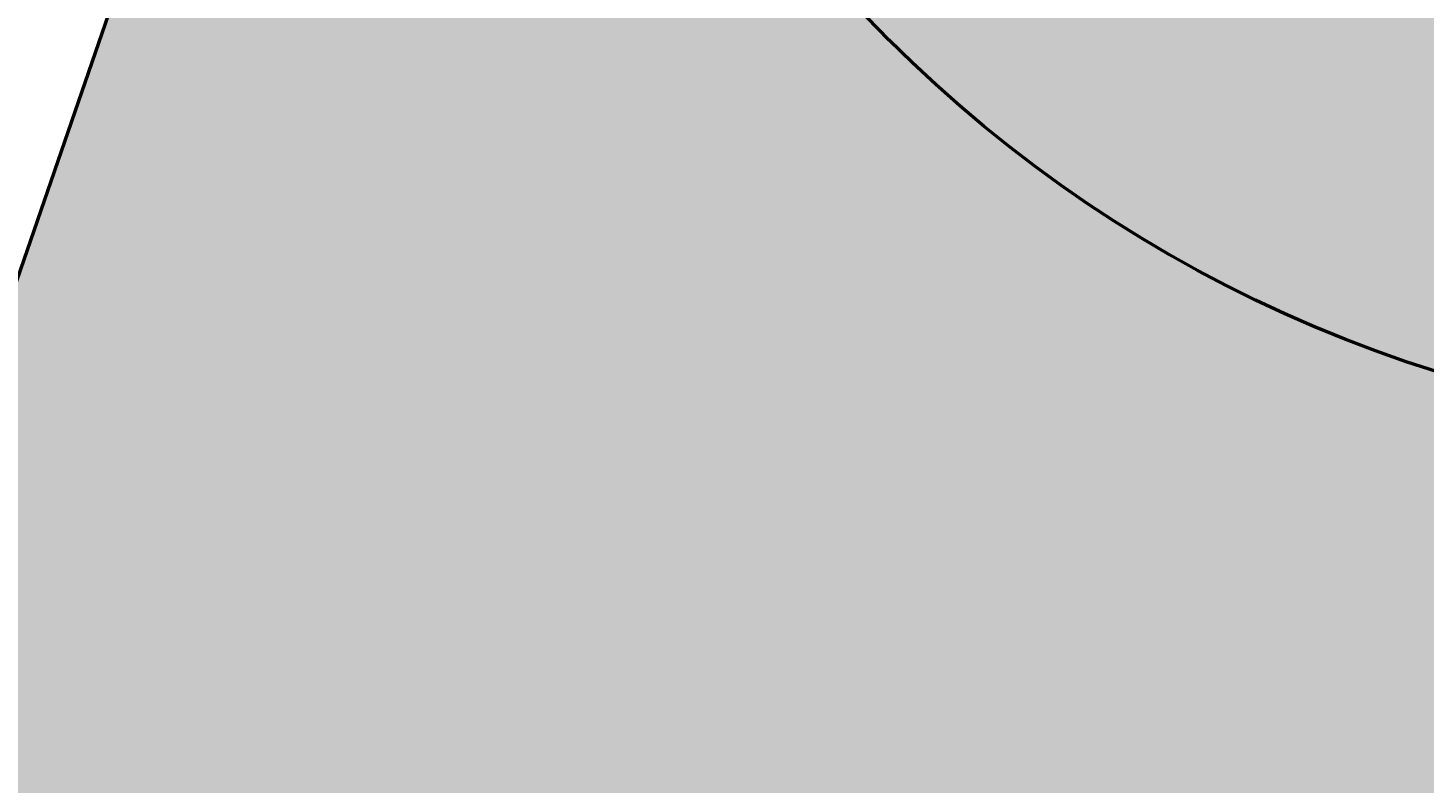
# Model space of a CAD drawing. Units: inches. Extents: x 114 to 236, y -51 to 115.
# Tile 6 of 14: x 135 to 166, y 41 to 58. Entities that reach past the tile are written whole.
import ezdxf

# ---------------------------------------------------------------- set-up
doc = ezdxf.new("R2010")
doc.units = ezdxf.units.IN
doc.header["$MEASUREMENT"] = 0
doc.layers.add('M-DIMS', color=2, linetype='Continuous', lineweight=18)
doc.layers.add('M-OUTL', color=7, linetype='Continuous', lineweight=50)
doc.layers.add('M-HATC', color=7, linetype='Continuous', lineweight=18, true_color=0xffffff)
doc.styles.get("Standard").update_dxf_attribs({"font": 'arial.ttf'})
doc.dimstyles.get("Standard").update_dxf_attribs({"dimtxt": 0.18, "dimasz": 0.18, "dimexe": 0.18, "dimexo": 0.0625, "dimgap": 0.09, "dimtad": 0, "dimtih": 1, "dimtoh": 1, "dimdec": 4, "dimzin": 0, "dimdsep": 46, "dimtxsty": 'Standard', "dimcen": 0.09, "dimadec": 0, "dimazin": 0, "dimtfac": 1, "dimtdec": 4, "dimtofl": 0, "dimtmove": 0, "dimatfit": 3, "dimfxl": 1, "dimtolj": 1, "dimtzin": 0, "dimarcsym": 0})

# ---------------------------------------------------------------- blocks, each defined once
blk = doc.blocks.new('*D3')
at = {"layer": 'Defpoints', "color": 0, "transparency": 16777216}
for p in [(230.229, 115.287), (120.229, 9.307), (230.229, 9.307)]:
    blk.add_point(p, dxfattribs=at)
at = {"layer": 'M-DIMS', "color": 0, "lineweight": -2, "transparency": 16777216}
for p, q in [((120.229, 9.37), (120.229, 115.467)), ((120.409, 115.287), (174.949, 115.287)), ((230.049, 115.287), (175.509, 115.287)), ((230.229, 9.37), (230.229, 115.467))]:
    blk.add_line(p, q, dxfattribs=at)
at = {"layer": 'M-DIMS', "color": 0, "transparency": 16777216}
for points in [[(120.409, 115.317), (120.409, 115.257), (120.229, 115.287)], [(230.049, 115.317), (230.049, 115.257), (230.229, 115.287)]]:
    blk.add_solid(points, dxfattribs=at)
at = {"layer": 'M-DIMS', "color": 0, "transparency": 16777216, "insert": (175.229, 115.287), "char_height": 0.18, "attachment_point": 5}
blk.add_mtext('\\A1;110', dxfattribs=at)
blk = doc.blocks.new('*D4')
at = {"layer": 'Defpoints', "color": 0, "transparency": 16777216}
for p in [(114.249, 109.307), (175.229, 109.307), (135.229, -5.693)]:
    blk.add_point(p, dxfattribs=at)
at = {"layer": 'M-DIMS', "color": 0, "lineweight": -2, "transparency": 16777216}
for p, q in [((175.166, 109.307), (114.069, 109.307)), ((114.249, 109.127), (114.249, 51.989)), ((114.249, -5.513), (114.249, 51.625)), ((135.166, -5.693), (114.069, -5.693))]:
    blk.add_line(p, q, dxfattribs=at)
at = {"layer": 'M-DIMS', "color": 0, "transparency": 16777216}
for points in [[(114.219, 109.127), (114.279, 109.127), (114.249, 109.307)], [(114.219, -5.513), (114.279, -5.513), (114.249, -5.693)]]:
    blk.add_solid(points, dxfattribs=at)
at = {"layer": 'M-DIMS', "color": 0, "transparency": 16777216, "insert": (114.249, 51.807), "char_height": 0.18, "attachment_point": 5}
blk.add_mtext('\\A1;115', dxfattribs=at)
blk = doc.blocks.new('*D5')
at = {"layer": 'Defpoints', "color": 0, "transparency": 16777216}
for p in [(175.229, 79.307), (135.229, 9.307), (175.229, -11.673)]:
    blk.add_point(p, dxfattribs=at)
at = {"layer": 'M-DIMS', "color": 0, "lineweight": -2, "transparency": 16777216}
for p, q in [((175.229, 79.245), (175.229, -11.853)), ((135.229, 9.245), (135.229, -11.853)), ((135.409, -11.673), (155.006, -11.673)), ((175.049, -11.673), (155.451, -11.673))]:
    blk.add_line(p, q, dxfattribs=at)
at = {"layer": 'M-DIMS', "color": 0, "transparency": 16777216}
for points in [[(135.409, -11.643), (135.409, -11.703), (135.229, -11.673)], [(175.049, -11.643), (175.049, -11.703), (175.229, -11.673)]]:
    blk.add_solid(points, dxfattribs=at)
at = {"layer": 'M-DIMS', "color": 0, "transparency": 16777216, "insert": (155.229, -11.673), "char_height": 0.18, "attachment_point": 5}
blk.add_mtext('\\A1;40', dxfattribs=at)

msp = doc.modelspace()

# ---------------------------------------------------------------- hatches: boundary and pattern name
at = {"layer": 'M-HATC'}
h = msp.add_hatch(color=256, dxfattribs=at)
h.set_gradient(color1=(19, 155, 72), color2=(255, 255, 0), tint=1, name='HEMISPHERICAL')
h.paths.add_polyline_path([(147.853, 91.577), (146.105, 86.505, 0.060651), (145.229, 79.307, 1), (205.229, 79.307, 0.060651), (204.352, 86.505), (202.605, 91.577, 0.647643)])
h.paths.add_polyline_path([(180.229, 99.307, -0.031342), (180.189, 98.682, -0.27393), (194.604, 84.268, -0.451416), (200.229, 79.307, -0.451416), (194.604, 74.346, -0.27393), (180.189, 59.932, -0.031342), (180.229, 59.307, -1), (170.229, 59.307, -0.031342), (170.268, 59.932, -0.27393), (155.854, 74.346, -0.451416), (150.229, 79.307, -0.451416), (155.854, 84.268, -0.27393), (170.268, 98.682, -0.031342), (170.229, 99.307, -1)], flags=16)
h.paths.add_polyline_path([(183.229, 79.307, -1), (167.229, 79.307, -1)], flags=0)
h.paths.add_polyline_path([(155.854, 84.268, -0.377964), (160.229, 79.307, -0.377964), (155.854, 74.346, 0.27393), (170.268, 59.932, -0.881917), (180.189, 59.932, 0.27393), (194.604, 74.346, -0.377964), (190.229, 79.307, -0.377964), (194.604, 84.268, 0.27393), (180.189, 98.682, -0.881917), (170.268, 98.682, 0.27393)], flags=0)
h = msp.add_hatch(color=256, dxfattribs=at)
h.set_gradient(color1=(242, 103, 34), color2=(255, 255, 0), tint=1, name='INVSPHERICAL')
h.paths.add_polyline_path([(145.229, 79.307, -0.060651), (146.105, 86.505), (121.823, 16.038, -0.790743), (150.229, 9.307, -0.236068), (144.229, -2.693, -0.14094), (175.229, 9.098, -0.14094), (206.229, -2.693, -0.236068), (200.229, 9.307, -0.790743), (228.634, 16.038), (204.352, 86.505, -0.060651), (205.229, 79.307, -1)])

# ---------------------------------------------------------------- linework, layer by layer
at = {"layer": 'M-OUTL'}
msp.add_line((120.523, 12.263), (147.853, 91.577), dxfattribs=at)
msp.add_circle((175.229, 79.307), 30, dxfattribs=at)

# ---------------------------------------------------------------- dimensions: what is measured, and where the dimension line sits
at = {"layer": 'M-DIMS'}
for base, p1, p2, picture, middle in [((230.229, 115.287), (120.229, 9.307), (230.229, 9.307), '*D3', (175.229, 115.287)), ((175.229, -11.673), (135.229, 9.307), (175.229, 79.307), '*D5', (155.229, -11.673))]:
    dim = msp.add_linear_dim(base=base, p1=p1, p2=p2, dimstyle='Standard', override={"dimdec": 0, "dimlfac": 1, "dimrnd": 0, "dimzin": 0, "dimdsep": 46, "dimlunit": 2}, dxfattribs=at)
    dim.commit()
    dim.dimension.update_dxf_attribs({"geometry": picture, "text_midpoint": middle})
dim = msp.add_linear_dim(base=(114.249, 109.307), p1=(135.229, -5.693), p2=(175.229, 109.307), angle=90, dimstyle='Standard', override={"dimdec": 0, "dimlfac": 1, "dimrnd": 0, "dimzin": 0, "dimdsep": 46, "dimlunit": 2}, dxfattribs=at)
dim.commit()
dim.dimension.update_dxf_attribs({"geometry": '*D4', "text_midpoint": (114.249, 51.807)})

doc.saveas('drawing.dxf')
